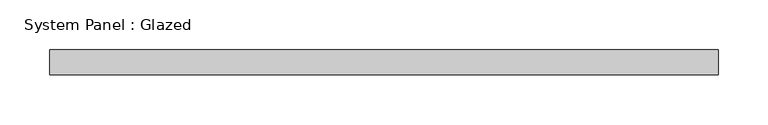
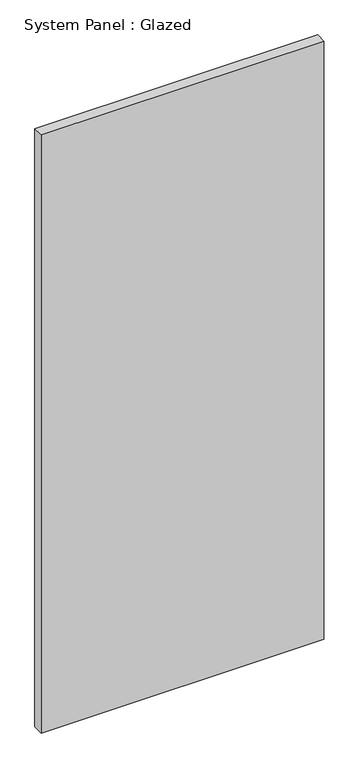
"""IFC4 building model written with IfcOpenShell, lengths in millimetres: plate geometry, System Panel : Glazed."""

from ifc_helpers import new_model, si_unit, origin, origin_with_axes, place, context, project, spatial, polyline, outline, extrude, source, transform, mapped, element, save


def system_panel_glazed_219b4c74(model_context):
    return source(origin(), model_context, "Body", "SweptSolid", [
        extrude(outline(polyline([(336.55, 19.05), (-336.55, 19.05), (-336.55, 44.45), (336.55, 44.45), (336.55, 19.05)])), origin_with_axes(), (0.0, 0.0, 1.0), 1506.7500384),
    ])


if __name__ == "__main__":
    model = new_model("IFC4")
    model_context = context("Model", 3, world=origin())
    ifc_project = project(units=[si_unit("LENGTHUNIT", "METRE", prefix="MILLI")], contexts=[model_context])
    site = spatial("IfcSite", under=ifc_project)
    building = spatial("IfcBuilding", under=site)
    placement = place(None, origin())
    system_panel_glazed_shape = system_panel_glazed_219b4c74(model_context)
    element("IfcPlate", 1, ObjectType="System Panel : Glazed", at=placement, inside=building, context=model_context, shape_type="MappedRepresentation", body=[
        mapped(system_panel_glazed_shape, transform((0.0, 0.0, 0.0), x_axis=(1.0, 0.0, 0.0), y_axis=(0.0, 1.0, 0.0), z_axis=(0.0, 0.0, 1.0))),
    ])
    save(model, "model.ifc")

# Revit data of these elements
# Type "System Panel : Glazed"
#   Construction Type Id = "GSP4R"
#   Analytic Construction = "1/8 in Pilkington single glazing"
#   Visual Light Transmittance = 0.9
#   Solar Heat Gain Coefficient = 0.86
#   Heat Transfer Coefficient (U) = 1.18115 BTU/(h·ft²·°F)
#   Define Thermal Properties by = 1
# Element 1 (IfcPlate, "System Panel : Glazed")
#   Materials on its faces: "Glass"
# Materials
#   "Glass": class "Glass", colour RGB 0 128 192, transparency 0.75, Description = "Soda Lime Glass", Cost = 0
